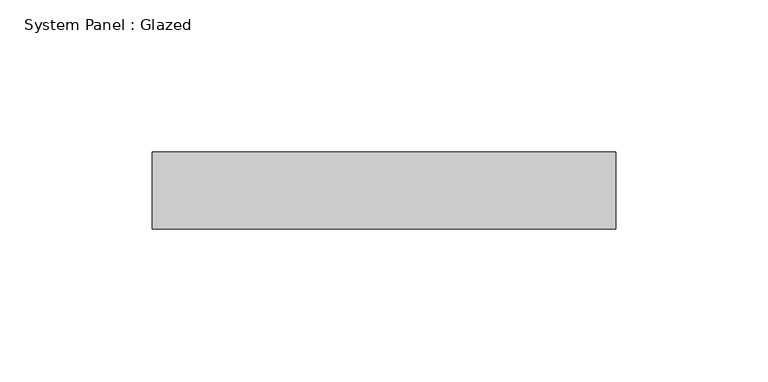
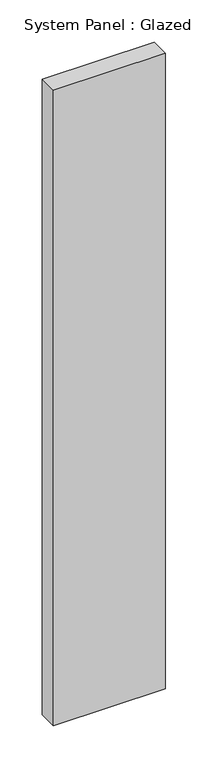
"""IFC4 building model written with IfcOpenShell, lengths in millimetres: plate geometry, System Panel : Glazed."""

from ifc_helpers import new_model, si_unit, origin, origin_with_axes, place, context, project, spatial, polyline, outline, extrude, source, transform, mapped, element, save


def system_panel_glazed_8df4d628(model_context):
    return source(origin(), model_context, "Body", "SweptSolid", [
        extrude(outline(polyline([(76.2, 19.05), (-76.2, 19.05), (-76.2, 44.45), (76.2, 44.45), (76.2, 19.05)])), origin_with_axes(), (0.0, 0.0, 1.0), 914.4),
    ])


if __name__ == "__main__":
    model = new_model("IFC4")
    model_context = context("Model", 3, world=origin())
    ifc_project = project(units=[si_unit("LENGTHUNIT", "METRE", prefix="MILLI")], contexts=[model_context])
    site = spatial("IfcSite", under=ifc_project)
    building = spatial("IfcBuilding", under=site)
    placement = place(None, origin())
    system_panel_glazed_shape = system_panel_glazed_8df4d628(model_context)
    element("IfcPlate", 1, ObjectType="System Panel : Glazed", at=placement, inside=building, context=model_context, shape_type="MappedRepresentation", body=[
        mapped(system_panel_glazed_shape, transform((0.0, 0.0, 0.0), x_axis=(1.0, 0.0, 0.0), y_axis=(0.0, 1.0, 0.0), z_axis=(0.0, 0.0, 1.0))),
    ])
    save(model, "model.ifc")

# Revit data of these elements
# Type "System Panel : Glazed"
#   Construction Type Id = "GSP4R"
#   Analytic Construction = "1/8 in Pilkington single glazing"
#   Visual Light Transmittance = 0.9
#   Solar Heat Gain Coefficient = 0.86
#   Heat Transfer Coefficient (U) = 1.18115 BTU/(h·ft²·°F)
# Element 1 (IfcPlate, "System Panel : Glazed")
#   Materials on its faces: "Glass"
# Materials
#   "Glass": class "Glass", colour RGB 0 128 192, transparency 0.75, Description = "Soda Lime Glass", Cost = 0
